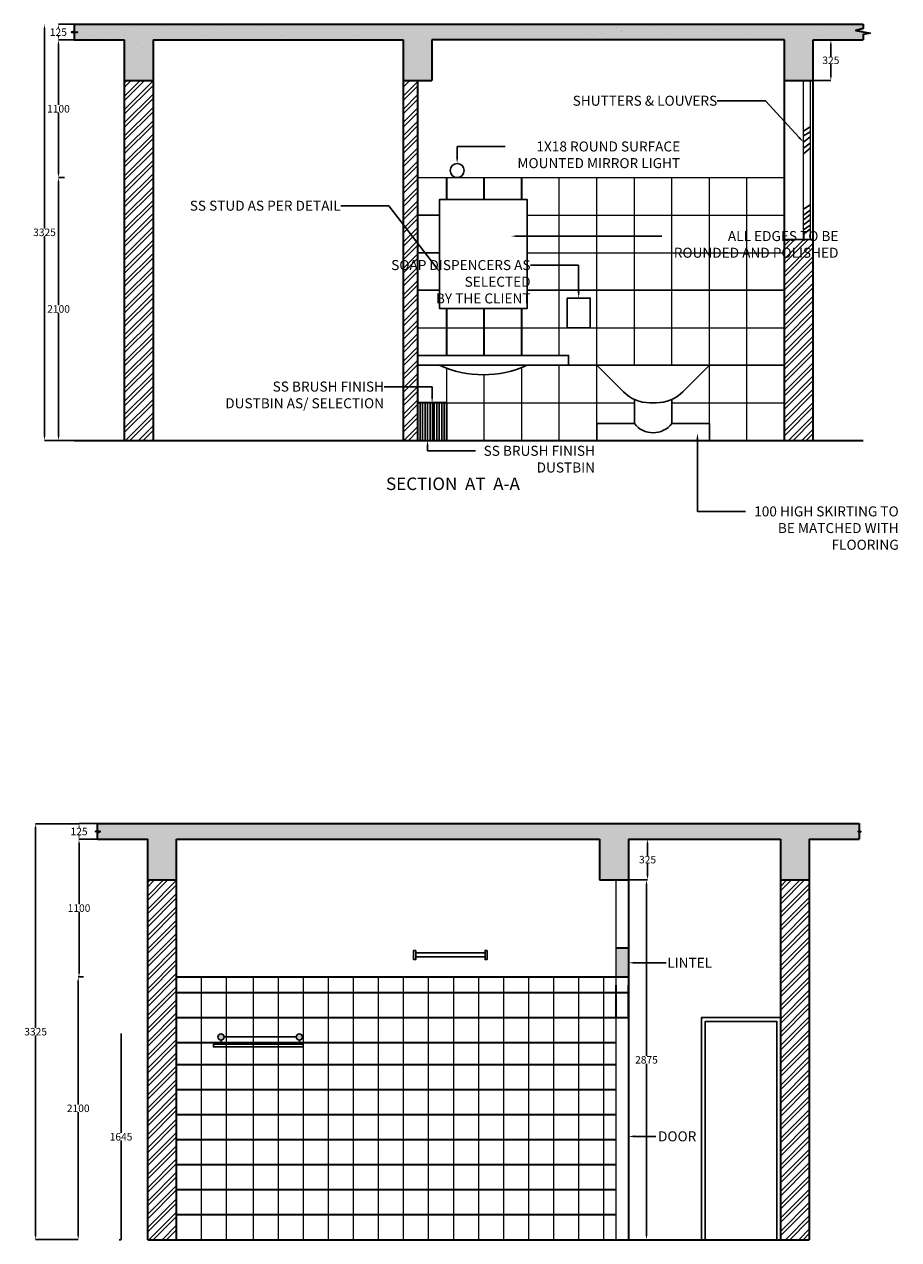
# Model space of a CAD drawing. Units: millimetres. Extents: x -2204 to 11247, y -2365 to 12631.
# Tile 3 of 3: x 4255 to 11247, y 2917 to 12631. Entities that reach past the tile are written whole.
import ezdxf
from ezdxf import colors
from ezdxf.entities.mleader import LeaderData, LeaderLine
from ezdxf.math import Vec2, Vec3

# ---------------------------------------------------------------- set-up
doc = ezdxf.new("R2010")
doc.units = ezdxf.units.MM
doc.header["$MEASUREMENT"] = 0
for name, color, linetype, lineweight in [('A-ANNO-DIMS', 2, 'Continuous', 18), ('A-ANNO-TEXT', 7, 'Continuous', 18), ('A-DOOR', 4, 'Continuous', 25), ('A-ELEV-PATT', 9, 'Continuous', 13), ('A-FLOR-FIXT', 8, 'Continuous', 25), ('A-GLAZ', 4, 'Continuous', 25), ('A-SECT', 7, 'Continuous', 35), ('A-SECT-PATT', 252, 'Continuous', 18), ('A-WALL-PATT', 8, 'Continuous', 18)]:
    doc.layers.add(name, color=color, linetype=linetype, lineweight=lineweight)
doc.styles.get("Standard").update_dxf_attribs({"font": 'arial.ttf'})
doc.dimstyles.get("Standard").update_dxf_attribs({"dimtxt": 60, "dimasz": 0.18, "dimexe": 0.18, "dimexo": 0.0625, "dimgap": 0.09, "dimtad": 0, "dimtih": 1, "dimtoh": 1, "dimdec": 0, "dimzin": 0, "dimdsep": 46, "dimtxsty": 'Standard', "dimcen": 0.09, "dimadec": 0, "dimazin": 0, "dimtfac": 1, "dimtdec": 0, "dimtofl": 0, "dimtmove": 0, "dimatfit": 3, "dimfxl": 1, "dimtolj": 1, "dimtzin": 0, "dimarcsym": 0})

# ---------------------------------------------------------------- blocks, each defined once
blk = doc.blocks.new('*D12')
at = {"layer": 'A-ANNO-DIMS', "color": 0, "lineweight": -2, "transparency": 16777216}
for p, q in [((9086, 6117.4), (9239.3, 6117.4)), ((9239.1, 6087.4), (9239.1, 5985.6)), ((9239.1, 5822.4), (9239.1, 5924.1)), ((9086, 5792.4), (9239.3, 5792.4))]:
    blk.add_line(p, q, dxfattribs=at)
at = {"layer": 'A-ANNO-DIMS', "color": 0, "transparency": 16777216}
for points in [[(9234.1, 6087.4), (9244.1, 6087.4), (9239.1, 6117.4)], [(9234.1, 5822.4), (9244.1, 5822.4), (9239.1, 5792.4)]]:
    blk.add_solid(points, dxfattribs=at)
at = {"layer": 'Defpoints', "color": 0, "transparency": 16777216}
for p in [(9085.9, 6117.4), (9085.9, 5792.4), (9239.1, 5792.4)]:
    blk.add_point(p, dxfattribs=at)
at = {"layer": 'A-ANNO-DIMS', "color": 0, "transparency": 16777216, "insert": (9239.1, 5954.9), "char_height": 60, "attachment_point": 5}
blk.add_mtext('\\A1;325', dxfattribs=at)
blk = doc.blocks.new('*D13')
at = {"layer": 'A-ANNO-DIMS', "color": 0, "lineweight": -2, "transparency": 16777216}
for p, q in [((9239.1, 5792.6), (9230.1, 5792.6)), ((9230.3, 5762.6), (9230.3, 4385.7)), ((9230.3, 2947.4), (9230.3, 4324.2)), ((9239.1, 2917.4), (9230.1, 2917.4))]:
    blk.add_line(p, q, dxfattribs=at)
at = {"layer": 'A-ANNO-DIMS', "color": 0, "transparency": 16777216}
for points in [[(9225.3, 5762.6), (9235.3, 5762.6), (9230.3, 5792.6)], [(9225.3, 2947.4), (9235.3, 2947.4), (9230.3, 2917.4)]]:
    blk.add_solid(points, dxfattribs=at)
at = {"layer": 'Defpoints', "color": 0, "transparency": 16777216}
for p in [(9239.1, 5792.6), (9230.3, 2917.4), (9239.1, 2917.4)]:
    blk.add_point(p, dxfattribs=at)
at = {"layer": 'A-ANNO-DIMS', "color": 0, "transparency": 16777216, "insert": (9230.3, 4355), "char_height": 60, "attachment_point": 5}
blk.add_mtext('\\A1;2875', dxfattribs=at)
blk = doc.blocks.new('*D14')
at = {"layer": 'A-ANNO-DIMS', "color": 0, "lineweight": -2, "transparency": 16777216}
for p, q in [((4841.7, 6242.4), (4692.8, 6242.4)), ((4693, 6212.4), (4693, 6210.6)), ((4693, 6147.4), (4693, 6149.1)), ((4841.7, 6117.4), (4692.8, 6117.4))]:
    blk.add_line(p, q, dxfattribs=at)
at = {"layer": 'A-ANNO-DIMS', "color": 0, "transparency": 16777216}
for points in [[(4688, 6212.4), (4698, 6212.4), (4693, 6242.4)], [(4688, 6147.4), (4698, 6147.4), (4693, 6117.4)]]:
    blk.add_solid(points, dxfattribs=at)
at = {"layer": 'Defpoints', "color": 0, "transparency": 16777216}
for p in [(4693, 6242.4), (4841.7, 6242.4), (4841.7, 6117.4)]:
    blk.add_point(p, dxfattribs=at)
at = {"layer": 'A-ANNO-DIMS', "color": 0, "transparency": 16777216, "insert": (4693, 6179.9), "char_height": 60, "attachment_point": 5}
blk.add_mtext('\\A1;125', dxfattribs=at)
blk = doc.blocks.new('*D19')
at = {"layer": 'A-ANNO-DIMS', "color": 0, "lineweight": -2, "transparency": 16777216}
for p, q in [((4692.8, 6117.4), (4692.4, 6117.4)), ((4692.6, 6087.4), (4692.6, 5598.1)), ((4692.6, 5047.4), (4692.6, 5536.6)), ((4729.3, 5017.4), (4692.4, 5017.4))]:
    blk.add_line(p, q, dxfattribs=at)
at = {"layer": 'A-ANNO-DIMS', "color": 0, "transparency": 16777216}
for points in [[(4687.6, 6087.4), (4697.6, 6087.4), (4692.6, 6117.4)], [(4687.6, 5047.4), (4697.6, 5047.4), (4692.6, 5017.4)]]:
    blk.add_solid(points, dxfattribs=at)
at = {"layer": 'Defpoints', "color": 0, "transparency": 16777216}
for p in [(4692.6, 6117.4), (4692.8, 6117.4), (4729.4, 5017.4)]:
    blk.add_point(p, dxfattribs=at)
at = {"layer": 'A-ANNO-DIMS', "color": 0, "transparency": 16777216, "insert": (4692.6, 5567.4), "char_height": 60, "attachment_point": 5}
blk.add_mtext('\\A1;1100', dxfattribs=at)
blk = doc.blocks.new('*D20')
at = {"layer": 'A-ANNO-DIMS', "color": 0, "lineweight": -2, "transparency": 16777216}
for p, q in [((4692.6, 5017.4), (4686.2, 5017.4)), ((4686.3, 4987.4), (4686.3, 3998.1)), ((4686.3, 2947.4), (4686.3, 3936.6)), ((4686.4, 2917.4), (4686.5, 2917.4))]:
    blk.add_line(p, q, dxfattribs=at)
at = {"layer": 'A-ANNO-DIMS', "color": 0, "transparency": 16777216}
for points in [[(4681.3, 4987.4), (4691.3, 4987.4), (4686.3, 5017.4)], [(4681.3, 2947.4), (4691.3, 2947.4), (4686.3, 2917.4)]]:
    blk.add_solid(points, dxfattribs=at)
at = {"layer": 'Defpoints', "color": 0, "transparency": 16777216}
for p in [(4692.6, 5017.4), (4686.3, 2917.4), (4686.3, 2917.4)]:
    blk.add_point(p, dxfattribs=at)
at = {"layer": 'A-ANNO-DIMS', "color": 0, "transparency": 16777216, "insert": (4686.3, 3967.4), "char_height": 60, "attachment_point": 5}
blk.add_mtext('\\A1;2100', dxfattribs=at)
blk = doc.blocks.new('*D21')
at = {"layer": 'A-ANNO-DIMS', "color": 0, "lineweight": -2, "transparency": 16777216}
for p, q in [((4692.9, 6242.2), (4345.8, 6242.2)), ((4346, 6212.2), (4346, 4610.6)), ((4346, 2947.6), (4346, 4549.1)), ((4686.3, 2917.6), (4345.8, 2917.6))]:
    blk.add_line(p, q, dxfattribs=at)
at = {"layer": 'A-ANNO-DIMS', "color": 0, "transparency": 16777216}
for points in [[(4341, 6212.2), (4351, 6212.2), (4346, 6242.2)], [(4341, 2947.6), (4351, 2947.6), (4346, 2917.6)]]:
    blk.add_solid(points, dxfattribs=at)
at = {"layer": 'Defpoints', "color": 0, "transparency": 16777216}
for p in [(4346, 6242.2), (4693, 6242.2), (4686.3, 2917.6)]:
    blk.add_point(p, dxfattribs=at)
at = {"layer": 'A-ANNO-DIMS', "color": 0, "transparency": 16777216, "insert": (4346, 4579.9), "char_height": 60, "attachment_point": 5}
blk.add_mtext('\\A1;3325', dxfattribs=at)
blk = doc.blocks.new('*D22')
at = {"layer": 'A-ANNO-DIMS', "color": 0, "lineweight": -2, "transparency": 16777216}
for p, q in [((5026, 4562.4), (5028.9, 4562.4)), ((5028.7, 4562.2), (5028.7, 3770.6)), ((5028.7, 2917.6), (5028.7, 3709.1)), ((5012.6, 2917.4), (5028.9, 2917.4))]:
    blk.add_line(p, q, dxfattribs=at)
at = {"layer": 'A-ANNO-DIMS', "color": 0, "transparency": 16777216}
for points in [[(5028.6, 4562.2), (5028.7, 4562.2), (5028.7, 4562.4)], [(5028.6, 2917.6), (5028.7, 2917.6), (5028.7, 2917.4)]]:
    blk.add_solid(points, dxfattribs=at)
at = {"layer": 'Defpoints', "color": 0, "transparency": 16777216}
for p in [(5026, 4562.4), (5012.5, 2917.4), (5028.7, 2917.4)]:
    blk.add_point(p, dxfattribs=at)
at = {"layer": 'A-ANNO-DIMS', "color": 0, "transparency": 16777216, "insert": (5028.7, 3739.9), "char_height": 60, "attachment_point": 5}
blk.add_mtext('\\A1;1645', dxfattribs=at)
blk = doc.blocks.new('*D23')
at = {"layer": 'A-ANNO-DIMS', "color": 0, "lineweight": -2, "transparency": 16777216}
for p, q in [((4654.4, 12631), (4527.5, 12631)), ((4527.6, 12601), (4527.6, 12599.2)), ((4527.6, 12536), (4527.6, 12537.7)), ((4654.4, 12506), (4527.5, 12506))]:
    blk.add_line(p, q, dxfattribs=at)
at = {"layer": 'A-ANNO-DIMS', "color": 0, "transparency": 16777216}
for points in [[(4522.6, 12601), (4532.6, 12601), (4527.6, 12631)], [(4522.6, 12536), (4532.6, 12536), (4527.6, 12506)]]:
    blk.add_solid(points, dxfattribs=at)
at = {"layer": 'Defpoints', "color": 0, "transparency": 16777216}
for p in [(4527.6, 12631), (4654.4, 12631), (4654.4, 12506)]:
    blk.add_point(p, dxfattribs=at)
at = {"layer": 'A-ANNO-DIMS', "color": 0, "transparency": 16777216, "insert": (4527.6, 12568.5), "char_height": 60, "attachment_point": 5}
blk.add_mtext('\\A1;125', dxfattribs=at)
blk = doc.blocks.new('*D24')
at = {"layer": 'A-ANNO-DIMS', "color": 0, "lineweight": -2, "transparency": 16777216}
for p, q in [((10563.2, 12506), (10705, 12506)), ((10704.8, 12476), (10704.8, 12374.2)), ((10704.8, 12211), (10704.8, 12312.7)), ((10563.2, 12181), (10705, 12181))]:
    blk.add_line(p, q, dxfattribs=at)
at = {"layer": 'A-ANNO-DIMS', "color": 0, "transparency": 16777216}
for points in [[(10699.8, 12476), (10709.8, 12476), (10704.8, 12506)], [(10699.8, 12211), (10709.8, 12211), (10704.8, 12181)]]:
    blk.add_solid(points, dxfattribs=at)
at = {"layer": 'Defpoints', "color": 0, "transparency": 16777216}
for p in [(10563.2, 12506), (10563.2, 12181), (10704.8, 12181)]:
    blk.add_point(p, dxfattribs=at)
at = {"layer": 'A-ANNO-DIMS', "color": 0, "transparency": 16777216, "insert": (10704.8, 12343.5), "char_height": 60, "attachment_point": 5}
blk.add_mtext('\\A1;325', dxfattribs=at)
blk = doc.blocks.new('*D25')
at = {"layer": 'A-ANNO-DIMS', "color": 0, "lineweight": -2, "transparency": 16777216}
for p, q in [((4576.1, 12506), (4527.8, 12506)), ((4528, 12476), (4528, 11986.7)), ((4528, 11436), (4528, 11925.2)), ((4576.1, 11406), (4527.8, 11406))]:
    blk.add_line(p, q, dxfattribs=at)
at = {"layer": 'A-ANNO-DIMS', "color": 0, "transparency": 16777216}
for points in [[(4523, 12476), (4533, 12476), (4528, 12506)], [(4523, 11436), (4533, 11436), (4528, 11406)]]:
    blk.add_solid(points, dxfattribs=at)
at = {"layer": 'Defpoints', "color": 0, "transparency": 16777216}
for p in [(4528, 12506), (4576.1, 12506), (4576.1, 11406)]:
    blk.add_point(p, dxfattribs=at)
at = {"layer": 'A-ANNO-DIMS', "color": 0, "transparency": 16777216, "insert": (4528, 11956), "char_height": 60, "attachment_point": 5}
blk.add_mtext('\\A1;1100', dxfattribs=at)
blk = doc.blocks.new('*D26')
at = {"layer": 'A-ANNO-DIMS', "color": 0, "lineweight": -2, "transparency": 16777216}
for p, q in [((4576.1, 11406), (4529.1, 11406)), ((4529.3, 11376), (4529.3, 10386.7)), ((4529.3, 9336), (4529.3, 10325.2)), ((4654.4, 9306), (4529.1, 9306))]:
    blk.add_line(p, q, dxfattribs=at)
at = {"layer": 'A-ANNO-DIMS', "color": 0, "transparency": 16777216}
for points in [[(4524.3, 11376), (4534.3, 11376), (4529.3, 11406)], [(4524.3, 9336), (4534.3, 9336), (4529.3, 9306)]]:
    blk.add_solid(points, dxfattribs=at)
at = {"layer": 'Defpoints', "color": 0, "transparency": 16777216}
for p in [(4529.3, 11406), (4576.1, 11406), (4654.4, 9306)]:
    blk.add_point(p, dxfattribs=at)
at = {"layer": 'A-ANNO-DIMS', "color": 0, "transparency": 16777216, "insert": (4529.3, 10356), "char_height": 60, "attachment_point": 5}
blk.add_mtext('\\A1;2100', dxfattribs=at)
blk = doc.blocks.new('*D27')
at = {"layer": 'A-ANNO-DIMS', "color": 0, "lineweight": -2, "transparency": 16777216}
for p, q in [((4416.8, 12631), (4416.5, 12631)), ((4416.7, 12601), (4416.7, 10999.2)), ((4416.7, 9336), (4416.7, 10937.7)), ((4529.1, 9306), (4416.5, 9306))]:
    blk.add_line(p, q, dxfattribs=at)
at = {"layer": 'A-ANNO-DIMS', "color": 0, "transparency": 16777216}
for points in [[(4411.7, 12601), (4421.7, 12601), (4416.7, 12631)], [(4411.7, 9336), (4421.7, 9336), (4416.7, 9306)]]:
    blk.add_solid(points, dxfattribs=at)
at = {"layer": 'Defpoints', "color": 0, "transparency": 16777216}
for p in [(4416.8, 12631), (4416.7, 9306), (4529.1, 9306)]:
    blk.add_point(p, dxfattribs=at)
at = {"layer": 'A-ANNO-DIMS', "color": 0, "transparency": 16777216, "insert": (4416.7, 10968.5), "char_height": 60, "attachment_point": 5}
blk.add_mtext('\\A1;3325', dxfattribs=at)

msp = doc.modelspace()

# ---------------------------------------------------------------- hatches: boundary and pattern name
at = {"layer": 'A-FLOR-FIXT'}
h = msp.add_hatch(color=256, dxfattribs=at)
h.dxf.hatch_style = 1
h.paths.add_polyline_path([(6430, 4537.4, 1), (6479.9, 4537.4, 1)])
h.paths.add_polyline_path([(5803.9, 4537.4, 1), (5853.8, 4537.4, 1)])
at = {"layer": 'A-SECT-PATT'}
h = msp.add_hatch(dxfattribs=at)
h.set_pattern_fill('AR-SAND', color=256, scale=200)
h.paths.add_polyline_path([(7514.4, 12506), (10333.2, 12506), (10333.2, 12181), (10563.2, 12181), (10563.2, 12506), (10963.2, 12506), (10963.2, 12631), (4654.4, 12631), (4654.4, 12506), (5054.4, 12506), (5054.4, 12181), (5284.4, 12181), (5284.4, 12506), (7284.4, 12506), (7284.4, 12181), (7514.4, 12181)])
h = msp.add_hatch(dxfattribs=at)
h.set_pattern_fill('AR-SAND', color=256, scale=200)
h.paths.add_polyline_path([(7514.4, 12506), (10333.2, 12506), (10333.2, 12181), (10563.2, 12181), (10563.2, 12506), (10963.2, 12506), (10963.2, 12631), (4654.4, 12631), (4654.4, 12506), (5054.4, 12506), (5054.4, 12181), (5284.4, 12181), (5284.4, 12506), (7284.4, 12506), (7284.4, 12181), (7514.4, 12181)])
h = msp.add_hatch(dxfattribs=at)
h.set_pattern_fill('AR-SAND', color=256, scale=15)
h.paths.add_polyline_path([(7514.4, 12506), (10333.2, 12506), (10333.2, 12181), (10563.2, 12181), (10563.2, 12506), (10963.2, 12506), (10963.2, 12631), (4654.4, 12631), (4654.4, 12506), (5054.4, 12506), (5054.4, 12181), (5284.4, 12181), (5284.4, 12506), (7284.4, 12506), (7284.4, 12181), (7514.4, 12181)])
h = msp.add_hatch(dxfattribs=at)
h.set_pattern_fill('AR-SAND', color=256, scale=10)
h.paths.add_polyline_path([(4841.7, 6242.4), (4841.7, 6117.4), (5241.7, 6117.4), (5241.7, 5792.4), (5471.7, 5792.4), (5471.7, 6117.4), (8855.9, 6117.4), (8855.9, 5792.4), (9085.9, 5792.4), (9085.9, 6117.4), (10302.2, 6117.4), (10302.2, 5792.4), (10532.2, 5792.4), (10532.2, 6117.4), (10932.2, 6117.4), (10932.2, 6242.4)])
h = msp.add_hatch(color=256, dxfattribs=at)
h.dxf.hatch_style = 1
h.paths.add_polyline_path([(9085.9, 5249.2), (8985.9, 5249.2), (8985.9, 5017.4), (9085.9, 5017.4)])
at = {"layer": 'A-WALL-PATT'}
h = msp.add_hatch(dxfattribs=at)
h.set_pattern_fill('ANSI32', color=256, scale=200)
h.paths.add_polyline_path([(5284.4, 12181), (5054.4, 12181), (5054.4, 9306), (5284.4, 9306)])
h = msp.add_hatch(dxfattribs=at)
h.set_pattern_fill('ANSI32', color=256, scale=200)
h.paths.add_polyline_path([(7399.4, 12181), (7284.4, 12181), (7284.4, 9306), (7399.4, 9306)])
h = msp.add_hatch(dxfattribs=at)
h.set_pattern_fill('ANSI32', color=256, scale=200)
h.paths.add_polyline_path([(10563.2, 10911.5), (10333.2, 10911.5), (10333.2, 9306), (10563.2, 9306)])
h = msp.add_hatch(dxfattribs=at)
h.set_pattern_fill('ANSI32', color=256, scale=200)
h.paths.add_polyline_path([(5241.7, 2917.4), (5471.7, 2917.4), (5471.7, 5792.4), (5241.7, 5792.4)])
h.paths.add_polyline_path([(10302.2, 2917.4), (10532.2, 2917.4), (10532.2, 5792.4), (10302.2, 5792.4)])

# ---------------------------------------------------------------- linework, layer by layer
at = {"layer": 'A-DOOR'}
msp.add_lwpolyline([(10302.2, 4692.4), (9669.7, 4692.4), (9669.7, 2917.4), (10302.2, 2917.4)], close=True, dxfattribs=at)
msp.add_lwpolyline([(10272.2, 2917.4), (10272.2, 4662.4), (9699.7, 4662.4), (9699.7, 2917.4)], dxfattribs=at)
at = {"layer": 'A-ELEV-PATT'}
for p, q in [((10485.4, 10911.5), (10485.4, 12181)), ((10538, 12181), (10538, 10911.5)), ((7399.4, 11406), (10333.2, 11406)), ((8533.2, 9985), (8533.2, 11406)), ((8833.2, 9306), (8833.2, 11406)), ((9133.2, 9906), (9133.2, 11406)), ((9433.2, 9906), (9433.2, 11406)), ((9733.2, 9306), (9733.2, 11406)), ((10033.2, 9306), (10033.2, 11406)), ((8275.8, 11106), (10333.2, 11106)), ((8275.8, 10806), (10333.2, 10806)), ((7399.4, 10206), (10333.2, 10206)), ((7633.2, 9306), (7633.2, 9882.5)), ((7933.2, 9306), (7933.2, 9829.9)), ((8233.2, 9306), (8233.2, 9887.9)), ((8533.2, 9306), (8533.2, 9906)), ((7399.4, 9606), (9133.2, 9606)), ((9433.2, 9606), (10333.2, 9606)), ((8985.9, 5792.4), (8985.9, 2917.4)), ((5671.7, 2917.4), (5671.7, 5017.4)), ((5871.7, 2917.4), (5871.7, 5017.4)), ((6085.9, 5017.4), (6085.9, 2917.4)), ((6285.9, 5017.4), (6285.9, 2917.4)), ((6485.9, 5017.4), (6485.9, 2917.4)), ((6685.9, 5017.4), (6685.9, 2917.4)), ((6885.9, 5017.4), (6885.9, 2917.4)), ((7085.9, 5017.4), (7085.9, 2917.4)), ((7285.9, 5017.4), (7285.9, 2917.4)), ((7485.9, 5017.4), (7485.9, 2917.4)), ((7685.9, 5017.4), (7685.9, 2917.4)), ((7885.9, 5017.4), (7885.9, 2917.4)), ((8085.9, 5017.4), (8085.9, 2917.4)), ((8285.9, 5017.4), (8285.9, 2917.4)), ((8485.9, 5017.4), (8485.9, 2917.4)), ((8685.9, 5017.4), (8685.9, 2917.4)), ((8885.9, 5017.4), (8885.9, 2917.4))]:
    msp.add_line(p, q, dxfattribs=at)
at = {"layer": 'A-FLOR-FIXT'}
for p, q in [((7399.4, 11106), (7576.3, 11106)), ((7399.4, 10806), (7576.3, 10806)), ((7399.4, 10506), (7576.3, 10506)), ((8275.8, 10506), (10333.2, 10506)), ((7399.4, 9906), (8833.2, 9906)), ((9045.3, 9693.8), (8833.2, 9906)), ((8833.2, 9906), (9733.2, 9906)), ((9521, 9693.8), (9733.2, 9906)), ((9733.2, 9906), (10333.2, 9906)), ((9133.2, 9440), (9133.2, 9632.9)), ((9433.2, 9440), (9433.2, 9632.9)), ((9257.4, 9606), (9308.9, 9606)), ((5829.2, 4481.1), (5829.2, 4512.4)), ((5853.8, 4537.4), (6430, 4537.4)), ((6454.9, 4481.1), (6454.9, 4512.4))]:
    msp.add_line(p, q, dxfattribs=at)
for points in [[(8275.8, 10506), (8275.8, 10359.4), (7576.3, 10359.4), (7576.3, 11231.5), (8275.8, 11231.5), (8275.8, 10506)], [(7419.4, 9606), (7419.4, 9306)], [(7439.4, 9606), (7439.4, 9306)], [(7459.4, 9606), (7459.4, 9306)], [(7479.4, 9606), (7479.4, 9306)], [(7499.4, 9606), (7499.4, 9306)], [(7519.4, 9606), (7519.4, 9306)], [(7533.2, 9306), (7533.2, 9606)], [(7553.2, 9306), (7553.2, 9606)], [(7573.2, 9306), (7573.2, 9606)], [(7593.2, 9306), (7593.2, 9606)], [(7613.2, 9306), (7613.2, 9606)], [(9133.2, 9440), (8833.2, 9440), (8833.2, 9306), (9733.2, 9306), (9733.2, 9440), (9433.2, 9440)]]:
    msp.add_lwpolyline(points, dxfattribs=at)
for points in [[(8595.2, 10443), (8780.7, 10443), (8780.7, 10206), (8595.2, 10206)], [(7399.4, 9906), (8607.1, 9906), (8607.1, 9985), (7399.4, 9985)], [(7384.7, 5229.2), (7367.9, 5229.2), (7367.9, 5156.7), (7384.7, 5156.7)], [(7384.7, 5210.5), (7939.6, 5210.5), (7939.6, 5179.3), (7384.7, 5179.3)], [(7956.3, 5229.2), (7939.6, 5229.2), (7939.6, 5156.7), (7956.3, 5156.7)], [(5766.9, 4481.1), (6485.9, 4481.1), (6485.9, 4458.3), (5766.9, 4458.3)]]:
    msp.add_lwpolyline(points, close=True, dxfattribs=at)
for centre, radius in [((7716.3, 11462.1), 56.2), ((5828.9, 4537.4), 25), ((6454.9, 4537.4), 25)]:
    msp.add_circle(centre, radius, dxfattribs=at)
for centre, radius, start, end in [((7926, 10671.7), 841.9, 245.45295, 294.54705), ((9257.4, 9906), 300, 225, 270), ((9308.9, 9906), 300, 270, 315), ((9283.2, 9557), 190.2, 217.9517, 322.0483)]:
    msp.add_arc(centre, radius, start, end, dxfattribs=at)
at = {"layer": 'A-GLAZ'}
for p, q in [((10485.4, 11777), (10538, 11811)), ((10485.4, 11739), (10538, 11770.9)), ((10485.4, 11688.7), (10538, 11731.2)), ((10485.4, 11641.2), (10538, 11682.4)), ((10485.4, 11596.6), (10538, 11641.1)), ((10485.4, 11154), (10538, 11187.8)), ((10485.4, 11106.9), (10538, 11146.8)), ((10485.4, 11068.8), (10538, 11110.1)), ((10485.4, 11028.6), (10538, 11069.6)), ((10485.4, 10988.9), (10538, 11027.1)), ((10485.4, 10953.1), (10538, 10994)), ((10333.2, 10911.5), (10563.2, 10911.5))]:
    msp.add_line(p, q, dxfattribs=at)
at = {"layer": 'A-SECT'}
for p, q in [((4654.4, 12631), (10963.2, 12631)), ((4654.4, 12631), (4654.4, 12573.2)), ((10963.2, 12631), (10963.2, 12596.8)), ((4654.4, 12563.3), (4654.4, 12506)), ((10963.2, 12550), (10963.2, 12506)), ((4654.4, 12506), (5054.4, 12506)), ((5054.4, 12506), (5054.4, 9306)), ((5284.4, 12506), (5284.4, 9306)), ((5284.4, 12506), (7284.4, 12506)), ((7284.4, 12506), (7284.4, 9306)), ((7514.4, 12506), (7514.4, 12181)), ((10333.2, 12506), (7514.4, 12506)), ((10333.2, 12181), (10333.2, 12506)), ((10563.2, 9306), (10563.2, 12506)), ((10563.2, 12506), (10963.2, 12506)), ((5054.4, 12181), (5284.4, 12181)), ((7284.4, 12181), (7514.4, 12181)), ((7399.4, 12181), (7399.4, 9306)), ((10333.2, 9306), (10333.2, 12181)), ((10333.2, 12181), (10563.2, 12181)), ((7633.2, 11231.5), (7633.2, 11406)), ((7933.2, 11231.5), (7933.2, 11406)), ((8233.2, 11231.5), (8233.2, 11406)), ((7633.2, 9985), (7633.2, 10359.4)), ((7933.2, 9985), (7933.2, 10359.4)), ((8233.2, 9985), (8233.2, 10359.4)), ((4654.4, 9306), (10963.2, 9306)), ((4841.7, 6242.4), (10932.2, 6242.4)), ((4841.7, 6188.2), (4841.7, 6242.4)), ((10932.2, 6242.4), (10932.2, 6187.7)), ((4841.7, 6117.4), (4841.7, 6171.9)), ((10932.2, 6172), (10932.2, 6117.4)), ((4841.7, 6117.4), (5241.7, 6117.4)), ((5241.7, 2917.4), (5241.7, 6117.4)), ((5471.7, 2917.4), (5471.7, 6117.4)), ((5471.7, 6117.4), (8855.9, 6117.4)), ((8855.9, 6117.4), (8855.9, 5792.4)), ((9085.9, 6117.4), (9085.9, 5792.4)), ((9085.9, 6117.4), (10302.2, 6117.4)), ((10302.2, 6117.4), (10302.2, 2917.4)), ((10532.2, 6117.4), (10532.2, 2917.4)), ((10532.2, 6117.4), (10932.2, 6117.4)), ((5241.7, 5792.4), (5471.7, 5792.4)), ((8855.9, 5792.4), (9085.9, 5792.4)), ((9085.9, 5792.4), (9085.9, 2917.4)), ((10302.2, 5792.4), (10532.2, 5792.4)), ((8985.9, 5249.2), (9085.9, 5249.2)), ((5471.7, 5017.4), (9085.9, 5017.4)), ((5471.7, 4892.4), (9085.9, 4892.4)), ((5471.7, 4692.4), (9085.9, 4692.4)), ((5471.7, 4492.4), (8985.9, 4492.4)), ((5471.7, 4317.4), (8985.9, 4317.4)), ((5471.7, 4117.4), (8985.9, 4117.4)), ((5471.7, 3917.4), (8985.9, 3917.4)), ((5471.7, 3717.4), (8985.9, 3717.4)), ((5471.7, 3517.4), (8985.9, 3517.4)), ((5471.7, 3317.4), (8985.9, 3317.4)), ((5471.7, 3117.4), (8985.9, 3117.4)), ((5241.7, 2917.4), (10532.2, 2917.4))]:
    msp.add_line(p, q, dxfattribs=at)
for points in [[(4654.4, 12631.1), (4654.4, 12573.2), (4631.8, 12568.6), (4679.7, 12568.3), (4654.4, 12563.3), (4654.4, 12511.9)], [(10963.2, 12631.1), (10963.2, 12596.8), (10903.3, 12580.5), (11017.7, 12559.1), (10963.2, 12550), (10963.2, 12505.8)], [(4841.7, 6117.2), (4841.7, 6171.9), (4862.8, 6179.7), (4824, 6180), (4841.7, 6188.2), (4841.7, 6242.6)], [(10932.2, 6242.6), (10932.2, 6187.7), (10922.5, 6180), (10943, 6179.7), (10932.2, 6172), (10932.2, 6117.2)], [(8985.9, 4951.4), (8985.9, 4692.4), (9085.9, 4692.4), (9085.9, 4951.4)]]:
    msp.add_lwpolyline(points, dxfattribs=at)
msp.add_lwpolyline([(7399.4, 9306), (7633.2, 9306), (7633.2, 9606), (7399.4, 9606)], close=True, dxfattribs=at)

# ---------------------------------------------------------------- texts
at = {"layer": 'A-ANNO-TEXT', "insert": (7147.7, 9008.8), "char_height": 100, "attachment_point": 1}
msp.add_mtext_dynamic_manual_height_columns('{\\fArial|b1|i0|c0|p34;SECTION  AT  A-A}', width=2816.974, gutter_width=1, heights=[0], dxfattribs=at)

# ---------------------------------------------------------------- dimensions: what is measured, and where the dimension line sits
at = {"layer": 'A-ANNO-DIMS'}
for base, p1, p2, override, picture, middle in [((4416.7, 9306), (4416.8, 12631), (4529.1, 9306), {"dimasz": 30, "dimclrd": 0, "dimclre": 0, "dimclrt": 0}, '*D27', (4416.7, 10968.5)), ((4527.6, 12631), (4654.4, 12506), (4654.4, 12631), {"dimasz": 30, "dimclrd": 0, "dimclre": 0, "dimclrt": 0}, '*D23', (4527.6, 12568.5)), ((4528, 12506), (4576.1, 11406), (4576.1, 12506), {"dimasz": 30, "dimclrd": 0, "dimclre": 0, "dimclrt": 0}, '*D25', (4528, 11956)), ((10704.8, 12181), (10563.2, 12506), (10563.2, 12181), {"dimasz": 30, "dimclrd": 0, "dimclre": 0, "dimclrt": 0}, '*D24', (10704.8, 12343.5)), ((4529.3, 11406), (4654.4, 9306), (4576.1, 11406), {"dimasz": 30, "dimclrd": 0, "dimclre": 0, "dimclrt": 0}, '*D26', (4529.3, 10356)), ((4346, 6242.2), (4686.3, 2917.6), (4693, 6242.2), {"dimasz": 30, "dimclrd": 0, "dimclre": 0, "dimclrt": 0}, '*D21', (4346, 4579.9)), ((4693, 6242.4), (4841.7, 6117.4), (4841.7, 6242.4), {"dimasz": 30, "dimclrd": 0, "dimclre": 0, "dimclrt": 0}, '*D14', (4693, 6179.9)), ((4692.6, 6117.4), (4729.4, 5017.4), (4692.8, 6117.4), {"dimasz": 30, "dimclrd": 0, "dimclre": 0, "dimclrt": 0}, '*D19', (4692.6, 5567.4)), ((9239.1, 5792.4), (9085.9, 6117.4), (9085.9, 5792.4), {"dimasz": 30, "dimclrd": 0, "dimclre": 0, "dimclrt": 0}, '*D12', (9239.1, 5954.9)), ((9230.3, 2917.4), (9239.1, 5792.6), (9239.1, 2917.4), {"dimasz": 30, "dimclrd": 0, "dimclre": 0, "dimclrt": 0}, '*D13', (9230.3, 4355)), ((4686.3, 2917.4), (4692.6, 5017.4), (4686.3, 2917.4), {"dimasz": 30, "dimclrd": 0, "dimclre": 0, "dimclrt": 0}, '*D20', (4686.3, 3967.4)), ((5028.7, 2917.4), (5026, 4562.4), (5012.5, 2917.4), {"dimclrd": 0, "dimclre": 0, "dimclrt": 0}, '*D22', (5028.7, 3739.9))]:
    dim = msp.add_linear_dim(base=base, p1=p1, p2=p2, angle=90, dimstyle='Standard', override=override, dxfattribs=at)
    dim.commit()
    dim.dimension.update_dxf_attribs({"geometry": picture, "text_midpoint": middle})

# ---------------------------------------------------------------- leaders
at = {"layer": 'A-ANNO-TEXT'}
ml = msp.add_multileader_mtext('Standard', dxfattribs=at)
ml.set_content('SHUTTERS & LOUVERS ', color=256)
ml.set_leader_properties()
ml.build(insert=Vec2(0, 0))
ml.multileader.update_dxf_attribs({"dogleg_length": 384.5, "arrow_head_size": 50})
ctx = ml.context
ctx.base_point, ctx.char_height, ctx.arrow_head_size, ctx.landing_gap_size, ctx.plane_origin = Vec3(8533.7, 12019.3), 80, 50, 0.09, Vec3(10485.4, 11688.7)
ctx.text_align_type = 2
notes = []
notes.append((ctx, [(0, (1, 1, 0), (10180.7, 12019.3), (-1, 0), 384.5, [(0, [(10485.4, 11688.7)], 0, [])])]))
ctx.mtext.insert, ctx.mtext.alignment, ctx.mtext.flow_direction = Vec3(9796, 12060.3), 3, 5
ml = msp.add_multileader_mtext('Standard', dxfattribs=at)
ml.set_content('1X18 ROUND SURFACE\\PMOUNTED MIRROR LIGHT', color=256)
ml.set_leader_properties()
ml.build(insert=Vec2(0, 0))
ml.multileader.update_dxf_attribs({"dogleg_length": 384.5, "arrow_head_size": 50})
ctx = ml.context
ctx.base_point, ctx.char_height, ctx.arrow_head_size, ctx.landing_gap_size, ctx.plane_origin = Vec3(8100.8, 11654.1), 80, 50, 0.09, Vec3(7716.3, 11518.3)
ctx.text_align_type = 2
notes.append((ctx, [(0, (1, 1, 0), (7716.3, 11654.1), (1, 0), 384.5, [(0, [(7716.3, 11518.3)], 0, [])])]))
ctx.mtext.insert, ctx.mtext.alignment, ctx.mtext.flow_direction = Vec3(9499.8, 11694.8), 3, 5
ml = msp.add_multileader_mtext('Standard', dxfattribs=at)
ml.set_content('SS STUD AS PER DETAIL ', color=256)
ml.set_leader_properties()
ml.build(insert=Vec2(0, 0))
ml.multileader.update_dxf_attribs({"dogleg_length": 384.5, "arrow_head_size": 50})
ctx = ml.context
ctx.base_point, ctx.char_height, ctx.arrow_head_size, ctx.landing_gap_size, ctx.plane_origin = Vec3(5447.8, 11180.8), 80, 50, 0.09, Vec3(7576.3, 10652)
ctx.text_align_type = 2
notes.append((ctx, [(0, (1, 1, 0), (7171.1, 11180.8), (-1, 0), 384.5, [(0, [(7576.3, 10652)], 0, [])])]))
ctx.mtext.insert, ctx.mtext.alignment, ctx.mtext.flow_direction = Vec3(6786.5, 11221.5), 3, 5
ml = msp.add_multileader_mtext('Standard', dxfattribs=at)
ml.set_content('ALL EDGES TO BE\\PROUNDED AND POLISHED', color=256)
ml.set_leader_properties()
ml.build(insert=Vec2(0, 0))
ml.multileader.update_dxf_attribs({"dogleg_length": 384.5, "arrow_head_size": 50})
ctx = ml.context
ctx.base_point, ctx.char_height, ctx.arrow_head_size, ctx.landing_gap_size, ctx.plane_origin = Vec3(9351.9, 10938.1), 80, 50, 0.09, Vec3(8148.8, 10938.1)
ctx.text_align_type = 2
notes.append((ctx, [(0, (1, 1, 0), (8967.4, 10938.1), (1, 0), 384.5, [(0, [(8148.8, 10938.1)], 0, [])])]))
ctx.mtext.insert, ctx.mtext.alignment, ctx.mtext.flow_direction = Vec3(10765.5, 10978.8), 3, 5
ml = msp.add_multileader_mtext('Standard', dxfattribs=at)
ml.set_content('SOAP DISPENCERS AS\\PSELECTED\\PBY THE CLIENT ', color=256)
ml.set_leader_properties()
ml.build(insert=Vec2(0, 0))
ml.multileader.update_dxf_attribs({"dogleg_length": 384.5, "arrow_head_size": 50})
ctx = ml.context
ctx.base_point, ctx.char_height, ctx.arrow_head_size, ctx.landing_gap_size, ctx.plane_origin = Vec3(7065.8, 10706.2), 80, 50, 0.09, Vec3(8688, 10443)
ctx.text_align_type = 2
notes.append((ctx, [(0, (1, 1, 0), (8688, 10706.2), (-1, 0), 384.5, [(0, [(8688, 10443)], 0, [])])]))
ctx.mtext.insert, ctx.mtext.alignment, ctx.mtext.flow_direction = Vec3(8303.4, 10746.9), 3, 5
ml = msp.add_multileader_mtext('Standard', dxfattribs=at)
ml.set_content('SS BRUSH FINISH \\PDUSTBIN AS/ SELECTION ', color=256)
ml.set_leader_properties()
ml.build(insert=Vec2(0, 0))
ml.multileader.update_dxf_attribs({"dogleg_length": 0.36, "arrow_head_size": 50})
ctx = ml.context
ctx.base_point, ctx.char_height, ctx.arrow_head_size, ctx.landing_gap_size, ctx.plane_origin = Vec3(5783.2, 9735), 80, 50, 0.09, Vec3(7516.3, 9606)
ctx.text_align_type = 2
notes.append((ctx, [(0, (1, 1, 0), (7516.3, 9735), (-1, 0), 384.5, [(0, [(7516.3, 9606)], 0, [])])]))
ctx.mtext.insert, ctx.mtext.alignment, ctx.mtext.flow_direction = Vec3(7131.7, 9775.7), 3, 5
ml = msp.add_multileader_mtext('Standard', dxfattribs=at)
ml.set_content('100 HIGH SKIRTING TO\\PBE MATCHED WITH\\PFLOORING', color=256)
ml.set_leader_properties()
ml.build(insert=Vec2(0, 0))
ml.multileader.update_dxf_attribs({"dogleg_length": 384.5, "arrow_head_size": 50})
ctx = ml.context
ctx.base_point, ctx.char_height, ctx.arrow_head_size, ctx.landing_gap_size, ctx.plane_origin = Vec3(10022.2, 8737.5), 80, 50, 0.09, Vec3(9637.7, 9362.9)
ctx.text_align_type = 2
notes.append((ctx, [(0, (1, 1, 0), (9637.7, 8737.5), (1, 0), 384.5, [(0, [(9637.7, 9362.9)], 0, [])])]))
ctx.mtext.insert, ctx.mtext.alignment, ctx.mtext.flow_direction = Vec3(11247.2, 8778.2), 3, 5
ml = msp.add_multileader_mtext('Standard', dxfattribs=at)
ml.set_content('SS BRUSH FINISH \\PDUSTBIN ', color=256)
ml.set_leader_properties()
ml.build(insert=Vec2(0, 0))
ml.multileader.update_dxf_attribs({"dogleg_length": 384.5, "arrow_head_size": 50})
ctx = ml.context
ctx.base_point, ctx.char_height, ctx.arrow_head_size, ctx.landing_gap_size, ctx.plane_origin = Vec3(7864, 9221.6), 80, 50, 0.09, Vec3(7479.4, 9306)
ctx.text_align_type = 2
notes.append((ctx, [(0, (1, 1, 0), (7479.4, 9221.6), (1, 0), 384.5, [(0, [(7479.4, 9306)], 0, [])])]))
ctx.mtext.insert, ctx.mtext.alignment, ctx.mtext.flow_direction = Vec3(8818.7, 9262.3), 3, 5
ml = msp.add_multileader_mtext('Standard', dxfattribs=at)
ml.set_content('LINTEL ', color=256)
ml.set_leader_properties()
ml.build(insert=Vec2(0, 0))
ml.multileader.update_dxf_attribs({"dogleg_length": 0.36, "arrow_head_size": 50})
ctx = ml.context
ctx.base_point, ctx.char_height, ctx.arrow_head_size, ctx.landing_gap_size, ctx.plane_origin = Vec3(9388.6, 5130.4), 80, 50, 0.09, Vec3(9085.9, 5130.4)
ctx.text_align_type = 2
notes.append((ctx, [(0, (1, 1, 0), (9388.2, 5130.4), (1, 0), 0.36, [(0, [(9085.9, 5130.4)], 0, [])])]))
ctx.mtext.insert, ctx.mtext.alignment, ctx.mtext.flow_direction = Vec3(9755.4, 5170.4), 3, 5
ml = msp.add_multileader_mtext('Standard', dxfattribs=at)
ml.set_content('DOOR ', color=256)
ml.set_leader_properties()
ml.build(insert=Vec2(0, 0))
ml.multileader.update_dxf_attribs({"dogleg_length": 0.36, "arrow_head_size": 50})
ctx = ml.context
ctx.base_point, ctx.char_height, ctx.arrow_head_size, ctx.landing_gap_size, ctx.plane_origin = Vec3(9303.7, 3742.7), 80, 50, 0.09, Vec3(9085.9, 3742.7)
ctx.text_align_type = 2
notes.append((ctx, [(0, (1, 1, 0), (9303.4, 3742.7), (1, 0), 0.36, [(0, [(9085.9, 3742.7)], 0, [])])]))
ctx.mtext.insert, ctx.mtext.alignment, ctx.mtext.flow_direction = Vec3(9629.1, 3783.4), 3, 5
for ctx, leaders in notes:
    for number, flags, end, landing, length, lines in leaders:
        leader = LeaderData()
        leader.index, (leader.has_last_leader_line, leader.has_dogleg_vector, leader.attachment_direction) = number, flags
        leader.last_leader_point, leader.dogleg_vector, leader.dogleg_length = Vec3(end), Vec3(landing), length
        for number, points, colour, breaks in lines:
            line = LeaderLine()
            line.index, line.vertices, line.color, line.breaks = number, Vec3.list(points), colors.encode_raw_color(colour), breaks
            leader.lines.append(line)
        ctx.leaders.append(leader)

doc.saveas('drawing.dxf')
